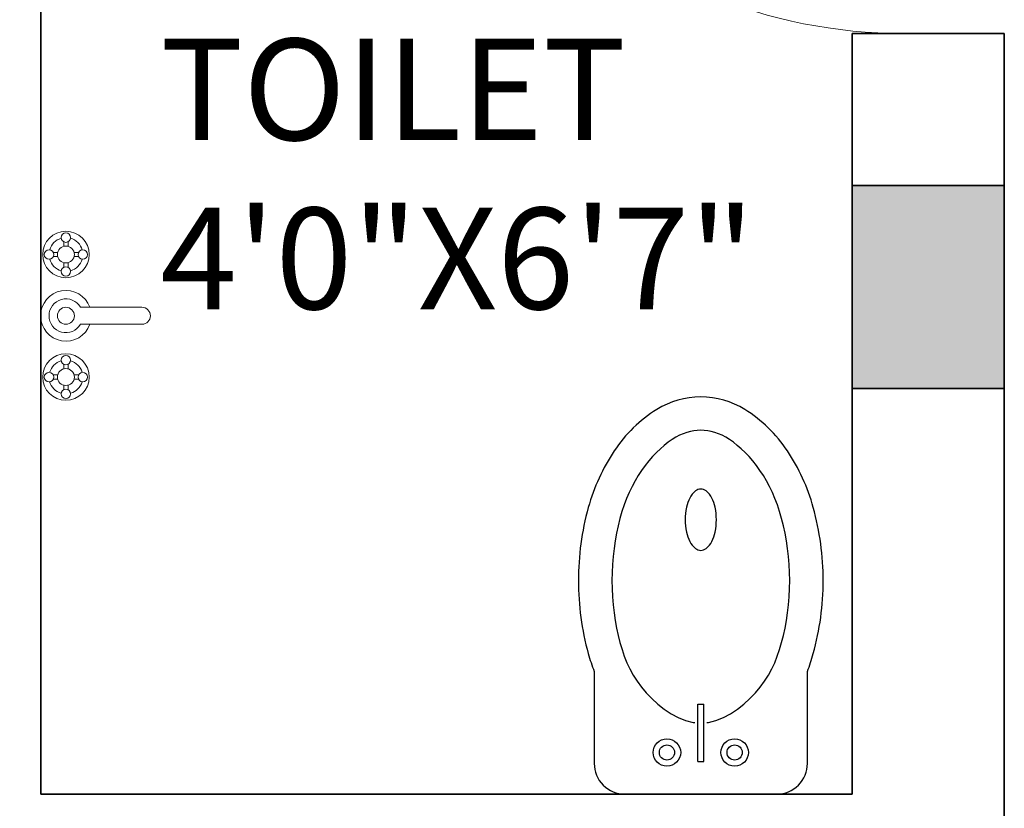
# Model space of a CAD drawing. Units: inches. Extents: x 3321 to 5237, y 11 to 1752.
# Tile 40 of 43: x 4943 to 5001, y 1598 to 1645. Entities that reach past the tile are written whole.
import ezdxf

# ---------------------------------------------------------------- set-up
doc = ezdxf.new("R2010")
doc.units = ezdxf.units.IN
for name, color, linetype, lineweight in [('A-ANNO-DIMS', 2, 'Continuous', 18), ('A-AREA-IDEN', 7, 'Continuous', 18), ('A-COLS', 1, 'Continuous', 35), ('A-DOOR', 4, 'Continuous', 18), ('A-WALL', 7, 'Continuous', 35), ('Сантехника', 7, 'Continuous', 18)]:
    doc.layers.add(name, color=color, linetype=linetype, lineweight=lineweight)
doc.layers.add('SANTEH', color=7, linetype='Continuous')
doc.styles.get("Standard").update_dxf_attribs({"font": 'arial.ttf'})
doc.dimstyles.new('ISO-25', dxfattribs={"dimtxt": 9, "dimasz": 2.5, "dimexe": 1.25, "dimexo": 0.625, "dimtad": 1, "dimdec": 1, "dimlunit": 3, "dimtxsty": 'Standard', "dimcen": 2.5, "dimclrd": 4, "dimclre": 4, "dimclrt": 256, "dimadec": 0, "dimazin": 0, "dimtfac": 1, "dimtdec": 1, "dimtmove": 0, "dimatfit": 3, "dimfxl": 1, "dimarcsym": 0})

# ---------------------------------------------------------------- blocks, each defined once
blk = doc.blocks.new('*U7')
for p, q in [((0, 0), (0, 6)), ((30, 0), (30, 6))]:
    blk.add_line(p, q)
blk.add_lwpolyline([(0, 0), (0, -30), (1.75, -30), (1.75, 0)], close=True)
blk.add_arc((0, 0), 30, 270, 0)
blk = doc.blocks.new('K10-45')
at = {"layer": 'SANTEH'}
for p, q in [((-18.9, 83.4), (-18.9, 177.1)), ((-18.9, 177.1), (-8.9, 177.1)), ((-8.9, 83.4), (-8.9, 177.1)), ((-18.9, 83.4), (-8.9, 83.4))]:
    blk.add_line(p, q, dxfattribs=at)
for points in [[(160.3, 230.4, 0.023928), (169.9, 259.6, 0.067459), (186.1, 379, 0.067459), (169.9, 498.4, 0.079812), (127.5, 591.1, 0.107118), (58, 658.5, 0.139889), (-13.9, 679, 0.139889), (-85.8, 658.5, 0.107118), (-155.3, 591.1, 0.079812), (-197.7, 498.4, 0.067459), (-213.9, 379, 0.067459), (-197.7, 259.6, 0.023928), (-188.1, 230.4), (-188.1, 80.2, 0.414214), (-138.1, 30.2), (110.3, 30.2, 0.414214), (160.3, 80.2)], [(-39.4, 478.5, 0.052061), (-37.3, 458.3, 0.065919), (-32, 443.1, 0.104629), (-22.6, 431.5, 0.172287), (-13.9, 428.4, 0.172287), (-5.2, 431.5, 0.104629), (4.1, 443.1, 0.065919), (9.5, 458.3, 0.052061), (11.6, 478.5, 0.052061), (9.5, 498.7, 0.065919), (4.1, 513.9, 0.104629), (-5.2, 525.5, 0.172287), (-13.9, 528.6, 0.172287), (-22.6, 525.5, 0.104629), (-32, 513.9, 0.065919), (-37.3, 498.7, 0.052061)]]:
    blk.add_lwpolyline(points, format="xyb", close=True, dxfattribs=at)
blk.add_lwpolyline([(-3.9, 147), (-1.4, 147.2), (10.9, 150.3), (23, 155.1), (34.7, 161.4), (45.9, 168.8), (56.5, 177.2), (66.3, 186.2), (75.2, 195.5), (83.2, 205), (90.3, 214.7), (96.5, 224.5), (102, 234.5), (106.9, 244.7), (111.1, 255.3), (114.8, 266.2), (118.1, 277.6), (121.1, 289.3), (123.7, 301.4), (126, 313.8), (127.9, 326.5), (129.3, 339.5), (130.4, 352.6), (131.1, 365.8), (131.3, 379), (131.1, 392.2), (130.4, 405.4), (129.3, 418.5), (127.9, 431.4), (126, 444.2), (123.7, 456.6), (121.1, 468.7), (118.1, 480.4), (114.8, 491.7), (111.2, 502.6), (107.3, 513.1), (103, 523.1), (98.4, 532.7), (93.5, 541.9), (88.3, 550.7), (82.8, 559.1), (77.1, 567.1), (71, 574.6), (64.9, 581.7), (58.5, 588.3), (52.1, 594.4), (45.7, 600), (39.3, 605), (33, 609.4), (26.9, 613.2), (20.8, 616.4), (14.9, 619), (9, 621.1), (3.2, 622.7), (-2.5, 623.8), (-8.2, 624.5), (-13.9, 624.7), (-19.6, 624.5), (-25.3, 623.8), (-31, 622.7), (-36.8, 621.1), (-42.7, 619), (-48.6, 616.4), (-54.7, 613.2), (-60.9, 609.4), (-67.2, 605), (-73.5, 600), (-80, 594.4), (-86.4, 588.3), (-92.7, 581.7), (-98.9, 574.6), (-104.9, 567.1), (-110.6, 559.1), (-116.1, 550.7), (-121.3, 541.9), (-126.2, 532.7), (-130.8, 523.1), (-135.1, 513.1), (-139, 502.6), (-142.7, 491.7), (-146, 480.4), (-148.9, 468.7), (-151.5, 456.6), (-153.8, 444.2), (-155.7, 431.4), (-157.2, 418.5), (-158.2, 405.4), (-158.9, 392.2), (-159.1, 379), (-158.9, 365.8), (-158.2, 352.6), (-157.2, 339.5), (-155.7, 326.5), (-153.8, 313.8), (-151.5, 301.4), (-148.9, 289.3), (-146, 277.6), (-142.6, 266.2), (-138.9, 255.3), (-134.7, 244.7), (-129.8, 234.5), (-124.4, 224.5), (-118.1, 214.7), (-111, 205), (-103.1, 195.5), (-94.1, 186.2), (-84.3, 177.2), (-73.7, 168.8), (-62.5, 161.4), (-50.8, 155.1), (-38.7, 150.3), (-26.4, 147.2), (-23.9, 147)], dxfattribs=at)
for centre, radius in [((-69.2, 98.1), 22.4), ((41.4, 98.1), 22.4), ((-69.2, 98.1), 12.4), ((41.4, 98.1), 12.4)]:
    blk.add_circle(centre, radius, dxfattribs=at)
blk = doc.blocks.new('Faucet - Bathroom top')
for p, q in [((-3.75, 0.4788), (-3.75, 0.75)), ((-3.5, 0.482), (-3.5, 0.75)), ((3.5, 0.4788), (3.5, 0.75)), ((3.75, 0.482), (3.75, 0.75)), ((-4.107, 0.125), (-4.375, 0.125)), ((-3.1461, 0.125), (-2.875, 0.125)), ((3.143, 0.125), (2.875, 0.125)), ((4.1039, 0.125), (4.375, 0.125)), ((-4.1039, -0.125), (-4.375, -0.125)), ((-3.75, -0.4821), (-3.75, -0.75)), ((-3.5, -0.4789), (-3.5, -0.75)), ((-3.143, -0.125), (-2.875, -0.125)), ((3.1461, -0.125), (2.875, -0.125)), ((3.5, -0.4821), (3.5, -0.75)), ((3.75, -0.4789), (3.75, -0.75)), ((4.107, -0.125), (4.375, -0.125)), ((-0.5, -0.8639), (-0.5, -4.5)), ((0.5, -4.5), (0.5, -0.8631))]:
    blk.add_line(p, q)
for centre, radius in [((-3.625, 0), 1.375), ((-3.625, 1), 0.2795), ((3.625, 0), 1.375), ((3.625, 1), 0.2795), ((-4.625, 0), 0.2795), ((-3.625, 0), 0.5), ((-2.625, 0), 0.2795), ((0, 0), 0.5), ((2.625, 0), 0.2795), ((3.625, 0), 0.5), ((4.625, 0), 0.2795), ((-3.625, -1), 0.2795), ((3.625, -1), 0.2795)]:
    blk.add_circle(centre, radius)
for centre, radius, start, end in [((0, 0), 1.5, 289.6514, 250.3603), ((-3.625, 0), 1, 105.2407, 164.2093), ((-3.625, 0), 1, 16.44125, 74.07887), ((0, 0), 1, 300.3431, 239.7554), ((3.625, 0), 1, 106.12, 164.0884), ((3.625, 0), 1, 16.23422, 73.90469), ((-3.625, 0), 1, 196.2342, 253.9047), ((-3.625, 0), 1, 286.12, 344.0884), ((3.625, 0), 1, 196.4413, 254.0789), ((3.625, 0), 1, 285.2407, 344.2093), ((0, -4.5), 0.5, 180, 0)]:
    blk.add_arc(centre, radius, start, end)
blk = doc.blocks.new('COL-9X12-FURN-PLAN')
h = blk.add_hatch(color=256)
h.dxf.hatch_style = 1
h.paths.add_polyline_path([(0, 12), (0, 0), (9, 0), (9, 12)])
blk.add_lwpolyline([(0, 0), (9, 0), (9, 12), (0, 12)], close=True)
blk = doc.blocks.new('*D201')
at = {"layer": 'A-ANNO-DIMS', "color": 4, "lineweight": -2, "transparency": 16777216}
for p, q in [((4943.459, 1678.339), (4940.467, 1678.339)), ((4941.717, 1675.839), (4941.717, 1665.058)), ((4943.459, 1662.558), (4940.467, 1662.558)), ((4941.717, 1662.558), (4941.717, 1563.124))]:
    blk.add_line(p, q, dxfattribs=at)
at = {"layer": 'A-ANNO-DIMS', "color": 4, "transparency": 16777216}
for points in [[(4941.3, 1675.839), (4942.134, 1675.839), (4941.717, 1678.339)], [(4941.3, 1665.058), (4942.134, 1665.058), (4941.717, 1662.558)]]:
    blk.add_solid(points, dxfattribs=at)
at = {"layer": 'Defpoints', "color": 0, "transparency": 16777216}
for p in [(4944.084, 1678.339), (4941.717, 1662.558), (4944.084, 1662.558)]:
    blk.add_point(p, dxfattribs=at)
at = {"layer": 'A-ANNO-DIMS', "transparency": 16777216, "insert": (4936.439, 1611.591), "char_height": 9, "attachment_point": 5, "rotation": 90}
blk.add_mtext('BASIN 1\'-4" TYP.', dxfattribs=at)

msp = doc.modelspace()

# ---------------------------------------------------------------- linework, layer by layer
at = {"layer": 'A-WALL'}
for p, q in [((4944.084, 1678.339), (4944.084, 1599.339)), ((5001.084, 1644.339), (4992.084, 1644.339)), ((4992.084, 1644.339), (4992.084, 1599.339)), ((5001.084, 1644.339), (5001.084, 1594.339)), ((4992.084, 1599.339), (4944.084, 1599.339))]:
    msp.add_line(p, q, dxfattribs=at)

# ---------------------------------------------------------------- block references
at = {"layer": 'A-COLS'}
msp.add_blockref('COL-9X12-FURN-PLAN', (4992.084, 1623.339), dxfattribs=at)
at = {"layer": 'A-DOOR', "rotation": 270}
msp.add_blockref('*U7', (4995.084, 1674.339), dxfattribs=at)
at = {"layer": 'Сантехника', "rotation": 90}
msp.add_blockref('Faucet - Bathroom top', (4945.569, 1627.636), dxfattribs=at)
at = {"layer": 'Сантехника', "xscale": 0.0362080263207385, "yscale": 0.0362080263207385, "zscale": 0.0362080263207385}
msp.add_blockref('K10-45', (4983.632, 1598.245), dxfattribs=at)

# ---------------------------------------------------------------- texts
at = {"layer": 'A-AREA-IDEN', "insert": (4951.151, 1644.029), "char_height": 6, "attachment_point": 1}
msp.add_mtext_dynamic_manual_height_columns('TOILET\\P4\'0"X6\'7"', width=97.3114, gutter_width=25, heights=[0], dxfattribs=at)

# ---------------------------------------------------------------- dimensions: what is measured, and where the dimension line sits
at = {"layer": 'A-ANNO-DIMS'}
dim = msp.add_linear_dim(base=(4941.717, 1662.558), p1=(4944.084, 1678.339), p2=(4944.084, 1662.558), angle=270, text='BASIN <> TYP.', dimstyle='ISO-25', override={"dimdec": 1, "dimlfac": 1, "dimrnd": 0, "dimzin": 1, "dimdsep": 46, "dimlunit": 4, "dimfrac": 2}, dxfattribs=at)
dim.commit()
dim.dimension.update_dxf_attribs({"geometry": '*D201', "text_midpoint": (4936.439, 1611.591)})

doc.saveas('drawing.dxf')
